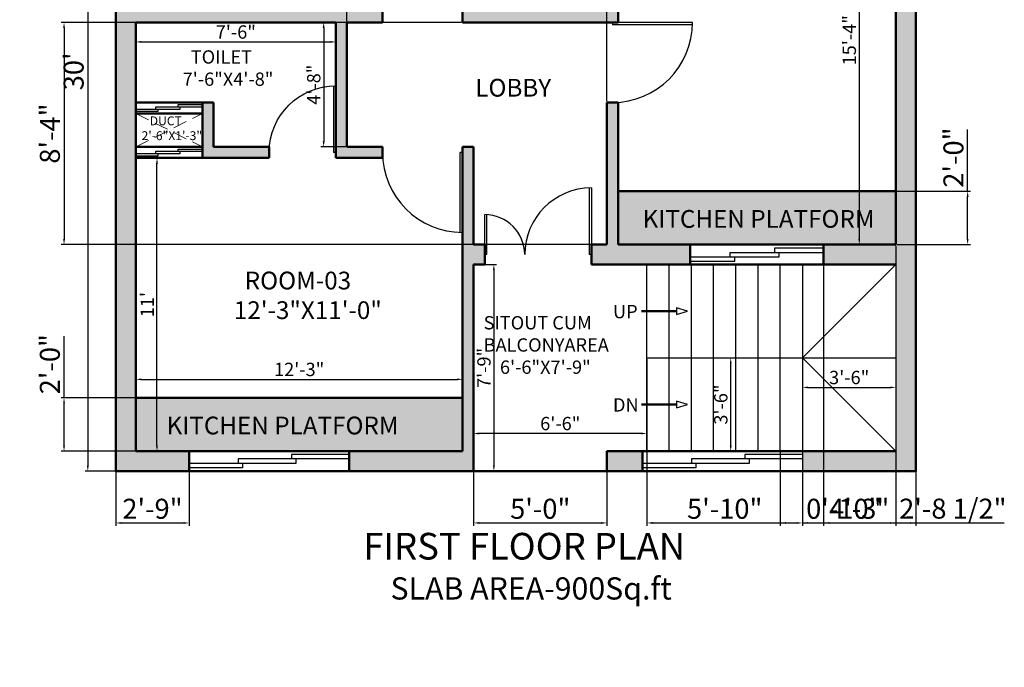
# Model space of a CAD drawing. Units: inches. Extents: x 3274 to 5176, y 1085 to 2172.
# Tile 15 of 16: x 4733 to 5176, y 1085 to 1377. Entities that reach past the tile are written whole.
import ezdxf

# ---------------------------------------------------------------- set-up
doc = ezdxf.new("R2010")
doc.units = ezdxf.units.IN
doc.linetypes.add('DASHED', pattern=[19.05, 12.7, -6.35])
for name, color, linetype, lineweight in [('A-ANNO-DIMS', 2, 'Continuous', 18), ('A-ANNO-TEXT', 7, 'Continuous', 25), ('A-AREA-IDEN', 3, 'Continuous', 25), ('A-DOOR', 4, 'Continuous', 25), ('A-FLOR-OPEN', 7, 'DASHED', 18), ('A-FLOR-PATT', 252, 'Continuous', 13), ('A-FLOR-STRS', 7, 'Continuous', 25), ('A-GLAZ', 5, 'Continuous', 25), ('A-WALL', 7, 'Continuous', 50), ('A-WALL-PATT', 8, 'Continuous', 13)]:
    doc.layers.add(name, color=color, linetype=linetype, lineweight=lineweight)
doc.styles.get("Standard").update_dxf_attribs({"font": 'arial.ttf'})
doc.dimstyles.new('ISO-25', dxfattribs={"dimtxt": 9, "dimasz": 2.5, "dimexe": 1.25, "dimexo": 0.625, "dimtad": 1, "dimdec": 1, "dimlunit": 3, "dimtxsty": 'Standard', "dimcen": 2.5, "dimclrd": 4, "dimclre": 4, "dimclrt": 1, "dimadec": 0, "dimazin": 0, "dimtfac": 1, "dimtdec": 1, "dimtmove": 0, "dimatfit": 3, "dimfxl": 1, "dimarcsym": 0})

# ---------------------------------------------------------------- blocks, each defined once
blk = doc.blocks.new('*D5')
at = {"layer": 'A-ANNO-DIMS', "color": 0, "lineweight": -2, "transparency": 16777216}
for p, q in [((4775.16, 1533.35), (4761.93, 1533.35)), ((4763.18, 1530.85), (4763.18, 1175.85)), ((4775.16, 1173.35), (4761.93, 1173.35))]:
    blk.add_line(p, q, dxfattribs=at)
at = {"layer": 'A-ANNO-DIMS', "color": 0, "transparency": 16777216}
for points in [[(4762.76, 1530.85), (4763.6, 1530.85), (4763.18, 1533.35)], [(4762.76, 1175.85), (4763.6, 1175.85), (4763.18, 1173.35)]]:
    blk.add_solid(points, dxfattribs=at)
at = {"layer": 'Defpoints', "color": 0, "transparency": 16777216}
for p in [(4775.78, 1533.35), (4763.18, 1173.35), (4775.78, 1173.35)]:
    blk.add_point(p, dxfattribs=at)
at = {"layer": 'A-ANNO-DIMS', "color": 0, "transparency": 16777216, "insert": (4757.96, 1353.35), "char_height": 9, "attachment_point": 5, "rotation": 90}
blk.add_mtext("30'", dxfattribs=at)
blk = doc.blocks.new('3')
for p, q in [((47, 30), (47, 0)), ((48, 30), (48, 0)), ((0, 0), (0, 18)), ((1, 0), (1, 18)), ((1, 0), (0, 0)), ((48, 0), (47, 0))]:
    blk.add_line(p, q)
for centre, radius, start, end in [((48, 0), 30, 90, 180), ((0, 0), 18, 0, 90)]:
    blk.add_arc(centre, radius, start, end)
blk = doc.blocks.new('1')
for p, q in [((0, 36), (0, 0)), ((1, 36), (1, 0)), ((0, 0), (1, 0))]:
    blk.add_line(p, q)
blk.add_arc((0, 0), 36, 0, 90)
blk = doc.blocks.new('2')
for p, q in [((0, 30), (0, 0)), ((1, 30), (1, 0)), ((0, 0), (1, 0))]:
    blk.add_line(p, q)
blk.add_arc((0, 0), 30, 0, 90)
blk = doc.blocks.new('*D89')
at = {"layer": 'A-ANNO-DIMS', "color": 0, "lineweight": -2, "transparency": 16777216}
for p, q in [((4784.78, 1206.98), (4784.78, 1215.95)), ((4787.28, 1214.7), (4929.28, 1214.7)), ((4931.78, 1206.98), (4931.78, 1215.95))]:
    blk.add_line(p, q, dxfattribs=at)
at = {"layer": 'A-ANNO-DIMS', "color": 0, "transparency": 16777216}
for points in [[(4787.28, 1215.11), (4787.28, 1214.28), (4784.78, 1214.7)], [(4929.28, 1215.11), (4929.28, 1214.28), (4931.78, 1214.7)]]:
    blk.add_solid(points, dxfattribs=at)
at = {"layer": 'Defpoints', "color": 0, "transparency": 16777216}
for p in [(4931.78, 1214.7), (4784.78, 1206.35), (4931.78, 1206.35)]:
    blk.add_point(p, dxfattribs=at)
at = {"layer": 'A-ANNO-DIMS', "color": 0, "transparency": 16777216, "insert": (4858.28, 1218.39), "char_height": 6, "attachment_point": 5}
blk.add_mtext('12\'-3"', dxfattribs=at)
blk = doc.blocks.new('*D90')
at = {"layer": 'A-ANNO-DIMS', "color": 0, "lineweight": -2, "transparency": 16777216}
for p, q in [((4785.41, 1314.35), (4795.56, 1314.35)), ((4794.31, 1184.85), (4794.31, 1311.85)), ((4785.41, 1182.35), (4795.56, 1182.35))]:
    blk.add_line(p, q, dxfattribs=at)
at = {"layer": 'A-ANNO-DIMS', "color": 0, "transparency": 16777216}
for points in [[(4793.89, 1311.85), (4794.72, 1311.85), (4794.31, 1314.35)], [(4793.89, 1184.85), (4794.72, 1184.85), (4794.31, 1182.35)]]:
    blk.add_solid(points, dxfattribs=at)
at = {"layer": 'Defpoints', "color": 0, "transparency": 16777216}
for p in [(4784.78, 1314.35), (4794.31, 1314.35), (4784.78, 1182.35)]:
    blk.add_point(p, dxfattribs=at)
at = {"layer": 'A-ANNO-DIMS', "color": 0, "transparency": 16777216, "insert": (4790.67, 1248.35), "char_height": 6, "attachment_point": 5, "rotation": 90}
blk.add_mtext("11'", dxfattribs=at)
blk = doc.blocks.new('*D91')
at = {"layer": 'A-ANNO-DIMS', "color": 0, "lineweight": -2, "transparency": 16777216}
for p, q in [((4784.78, 1374.73), (4784.78, 1365.34)), ((4874.78, 1374.73), (4874.78, 1365.34)), ((4787.28, 1366.59), (4872.28, 1366.59))]:
    blk.add_line(p, q, dxfattribs=at)
at = {"layer": 'A-ANNO-DIMS', "color": 0, "transparency": 16777216}
for points in [[(4787.28, 1367.01), (4787.28, 1366.18), (4784.78, 1366.59)], [(4872.28, 1367.01), (4872.28, 1366.18), (4874.78, 1366.59)]]:
    blk.add_solid(points, dxfattribs=at)
at = {"layer": 'Defpoints', "color": 0, "transparency": 16777216}
for p in [(4784.78, 1375.35), (4874.78, 1375.35), (4874.78, 1366.59)]:
    blk.add_point(p, dxfattribs=at)
at = {"layer": 'A-ANNO-DIMS', "color": 0, "transparency": 16777216, "insert": (4829.78, 1370.28), "char_height": 6, "attachment_point": 5}
blk.add_mtext('7\'-6"', dxfattribs=at)
blk = doc.blocks.new('*D92')
at = {"layer": 'A-ANNO-DIMS', "color": 0, "lineweight": -2, "transparency": 16777216}
for p, q in [((4874.16, 1375.35), (4868.06, 1375.35)), ((4869.31, 1372.85), (4869.31, 1321.85)), ((4879.16, 1319.35), (4868.06, 1319.35))]:
    blk.add_line(p, q, dxfattribs=at)
at = {"layer": 'A-ANNO-DIMS', "color": 0, "transparency": 16777216}
for points in [[(4868.89, 1372.85), (4869.73, 1372.85), (4869.31, 1375.35)], [(4868.89, 1321.85), (4869.73, 1321.85), (4869.31, 1319.35)]]:
    blk.add_solid(points, dxfattribs=at)
at = {"layer": 'Defpoints', "color": 0, "transparency": 16777216}
for p in [(4874.78, 1375.35), (4869.31, 1319.35), (4879.78, 1319.35)]:
    blk.add_point(p, dxfattribs=at)
at = {"layer": 'A-ANNO-DIMS', "color": 0, "transparency": 16777216, "insert": (4865.62, 1347.35), "char_height": 6, "attachment_point": 5, "rotation": 90}
blk.add_mtext('4\'-8"', dxfattribs=at)
blk = doc.blocks.new('*D98')
at = {"layer": 'A-ANNO-DIMS', "color": 0, "lineweight": -2, "transparency": 16777216}
for p, q in [((5091.41, 1459.35), (5111.56, 1459.35)), ((5110.31, 1456.85), (5110.31, 1277.85)), ((5091.41, 1275.35), (5111.56, 1275.35))]:
    blk.add_line(p, q, dxfattribs=at)
at = {"layer": 'A-ANNO-DIMS', "color": 0, "transparency": 16777216}
for points in [[(5109.9, 1456.85), (5110.73, 1456.85), (5110.31, 1459.35)], [(5109.9, 1277.85), (5110.73, 1277.85), (5110.31, 1275.35)]]:
    blk.add_solid(points, dxfattribs=at)
at = {"layer": 'Defpoints', "color": 0, "transparency": 16777216}
for p in [(5090.78, 1459.35), (5090.78, 1275.35), (5110.31, 1275.35)]:
    blk.add_point(p, dxfattribs=at)
at = {"layer": 'A-ANNO-DIMS', "color": 0, "transparency": 16777216, "insert": (5106.62, 1367.35), "char_height": 6, "attachment_point": 5, "rotation": 90}
blk.add_mtext('15\'-4"', dxfattribs=at)
blk = doc.blocks.new('*D104')
at = {"layer": 'A-ANNO-DIMS', "color": 0, "lineweight": -2, "transparency": 16777216}
for p, q in [((4937.41, 1266.35), (4947.14, 1266.35)), ((4945.89, 1263.85), (4945.89, 1175.85)), ((4937.41, 1173.35), (4947.14, 1173.35))]:
    blk.add_line(p, q, dxfattribs=at)
at = {"layer": 'A-ANNO-DIMS', "color": 0, "transparency": 16777216}
for points in [[(4945.48, 1263.85), (4946.31, 1263.85), (4945.89, 1266.35)], [(4945.48, 1175.85), (4946.31, 1175.85), (4945.89, 1173.35)]]:
    blk.add_solid(points, dxfattribs=at)
at = {"layer": 'Defpoints', "color": 0, "transparency": 16777216}
for p in [(4936.78, 1266.35), (4936.78, 1173.35), (4945.89, 1173.35)]:
    blk.add_point(p, dxfattribs=at)
at = {"layer": 'A-ANNO-DIMS', "color": 0, "transparency": 16777216, "insert": (4942.21, 1219.85), "char_height": 6, "attachment_point": 5, "rotation": 90}
blk.add_mtext('7\'-9"', dxfattribs=at)
blk = doc.blocks.new('*D105')
at = {"layer": 'A-ANNO-DIMS', "color": 0, "lineweight": -2, "transparency": 16777216}
for p, q in [((4936.78, 1190.96), (4936.78, 1191.58)), ((5012.28, 1190.33), (4939.28, 1190.33)), ((5014.78, 1190.96), (5014.78, 1191.58))]:
    blk.add_line(p, q, dxfattribs=at)
at = {"layer": 'A-ANNO-DIMS', "color": 0, "transparency": 16777216}
for points in [[(4939.28, 1190.75), (4939.28, 1189.92), (4936.78, 1190.33)], [(5012.28, 1190.75), (5012.28, 1189.92), (5014.78, 1190.33)]]:
    blk.add_solid(points, dxfattribs=at)
at = {"layer": 'Defpoints', "color": 0, "transparency": 16777216}
for p in [(4936.78, 1190.33), (4936.78, 1190.33), (5014.78, 1190.33)]:
    blk.add_point(p, dxfattribs=at)
at = {"layer": 'A-ANNO-DIMS', "color": 0, "transparency": 16777216, "insert": (4975.78, 1194.02), "char_height": 6, "attachment_point": 5}
blk.add_mtext('6\'-6"', dxfattribs=at)
blk = doc.blocks.new('*D106')
at = {"layer": 'A-ANNO-DIMS', "color": 0, "lineweight": -2, "transparency": 16777216}
for p, q in [((5050.97, 1224.35), (5053.72, 1224.35)), ((5052.47, 1184.85), (5052.47, 1221.85)), ((5050.97, 1182.35), (5053.72, 1182.35))]:
    blk.add_line(p, q, dxfattribs=at)
at = {"layer": 'A-ANNO-DIMS', "color": 0, "transparency": 16777216}
for points in [[(5052.06, 1221.85), (5052.89, 1221.85), (5052.47, 1224.35)], [(5052.06, 1184.85), (5052.89, 1184.85), (5052.47, 1182.35)]]:
    blk.add_solid(points, dxfattribs=at)
at = {"layer": 'Defpoints', "color": 0, "transparency": 16777216}
for p in [(5050.35, 1224.35), (5052.47, 1224.35), (5050.35, 1182.35)]:
    blk.add_point(p, dxfattribs=at)
at = {"layer": 'A-ANNO-DIMS', "color": 0, "transparency": 16777216, "insert": (5048.78, 1203.35), "char_height": 6, "attachment_point": 5, "rotation": 90}
blk.add_mtext('3\'-6"', dxfattribs=at)
blk = doc.blocks.new('*D107')
at = {"layer": 'A-ANNO-DIMS', "color": 0, "lineweight": -2, "transparency": 16777216}
for p, q in [((5084.78, 1213.78), (5084.78, 1209.81)), ((5087.28, 1211.06), (5124.28, 1211.06)), ((5126.78, 1213.78), (5126.78, 1209.81))]:
    blk.add_line(p, q, dxfattribs=at)
at = {"layer": 'A-ANNO-DIMS', "color": 0, "transparency": 16777216}
for points in [[(5087.28, 1211.47), (5087.28, 1210.64), (5084.78, 1211.06)], [(5124.28, 1211.47), (5124.28, 1210.64), (5126.78, 1211.06)]]:
    blk.add_solid(points, dxfattribs=at)
at = {"layer": 'Defpoints', "color": 0, "transparency": 16777216}
for p in [(5084.78, 1214.41), (5126.78, 1214.41), (5126.78, 1211.06)]:
    blk.add_point(p, dxfattribs=at)
at = {"layer": 'A-ANNO-DIMS', "color": 0, "transparency": 16777216, "insert": (5105.78, 1214.75), "char_height": 6, "attachment_point": 5}
blk.add_mtext('3\'-6"', dxfattribs=at)
blk = doc.blocks.new('WIN-30')
for p, q in [((4366.19, 1316.35), (4386.19, 1316.35)), ((4375.19, 1317.35), (4396.19, 1317.35)), ((4375.19, 1316.35), (4375.19, 1317.35)), ((4376.19, 1315.35), (4376.19, 1316.35)), ((4385.19, 1318.35), (4396.19, 1318.35)), ((4385.19, 1317.35), (4385.19, 1318.35)), ((4386.19, 1316.35), (4386.19, 1317.35)), ((4366.19, 1315.35), (4376.19, 1315.35))]:
    blk.add_line(p, q)
blk = doc.blocks.new('WIN-60')
for p, q in [((4598.19, 1271.85), (4640.19, 1271.85)), ((4598.19, 1269.85), (4598.19, 1271.85)), ((4618.19, 1273.85), (4640.19, 1273.85)), ((4618.19, 1271.85), (4618.19, 1273.85)), ((4620.19, 1269.85), (4620.19, 1271.85)), ((4580.19, 1269.85), (4620.19, 1269.85)), ((4580.19, 1267.85), (4600.19, 1267.85)), ((4600.19, 1267.85), (4600.19, 1269.85))]:
    blk.add_line(p, q)
blk = doc.blocks.new('WIN-72')
for p, q in [((4462.19, 1178.85), (4412.19, 1178.85)), ((4412.19, 1178.85), (4412.19, 1176.85)), ((4462.19, 1180.85), (4436.19, 1180.85)), ((4436.19, 1180.85), (4436.19, 1178.85)), ((4438.19, 1178.85), (4438.19, 1176.85)), ((4438.19, 1176.85), (4390.19, 1176.85)), ((4414.19, 1174.85), (4390.19, 1174.85)), ((4414.19, 1176.85), (4414.19, 1174.85))]:
    blk.add_line(p, q)
blk = doc.blocks.new('*D136')
at = {"layer": 'A-ANNO-DIMS', "color": 4, "lineweight": -2, "transparency": 16777216}
for p, q in [((4708.83, 1369.73), (4723.61, 1369.73)), ((4722.36, 1367.23), (4722.36, 1277.84)), ((4708.83, 1275.34), (4723.61, 1275.34)), ((4722.36, 1275.34), (4722.36, 1085.06))]:
    blk.add_line(p, q, dxfattribs=at)
at = {"layer": 'A-ANNO-DIMS', "color": 4, "transparency": 16777216}
for points in [[(4721.94, 1367.23), (4722.78, 1367.23), (4722.36, 1369.73)], [(4721.94, 1277.84), (4722.78, 1277.84), (4722.36, 1275.34)]]:
    blk.add_solid(points, dxfattribs=at)
at = {"layer": 'Defpoints', "color": 0, "transparency": 16777216}
for p in [(4708.2, 1369.73), (4708.2, 1275.34), (4722.36, 1275.34)]:
    blk.add_point(p, dxfattribs=at)
at = {"layer": 'A-ANNO-DIMS', "color": 1, "transparency": 16777216, "insert": (4717.08, 1178.95), "char_height": 9, "attachment_point": 5, "rotation": 90}
blk.add_mtext('L-SHAPED SOFA 7\'-10 1/2" TYP.', dxfattribs=at)
blk = doc.blocks.new('*D137')
at = {"layer": 'A-ANNO-DIMS', "color": 4, "lineweight": -2, "transparency": 16777216}
for p, q in [((4654.05, 1370.36), (4654.05, 1385.14)), ((4656.55, 1383.89), (4705.7, 1383.89)), ((4708.2, 1370.36), (4708.2, 1385.14)), ((4708.2, 1383.89), (4767.17, 1383.89))]:
    blk.add_line(p, q, dxfattribs=at)
at = {"layer": 'A-ANNO-DIMS', "color": 4, "transparency": 16777216}
for points in [[(4656.55, 1384.31), (4656.55, 1383.47), (4654.05, 1383.89)], [(4705.7, 1384.31), (4705.7, 1383.47), (4708.2, 1383.89)]]:
    blk.add_solid(points, dxfattribs=at)
at = {"layer": 'Defpoints', "color": 0, "transparency": 16777216}
for p in [(4708.2, 1383.89), (4654.05, 1369.73), (4708.2, 1369.73)]:
    blk.add_point(p, dxfattribs=at)
at = {"layer": 'A-ANNO-DIMS', "color": 1, "transparency": 16777216, "insert": (4738.94, 1389.11), "char_height": 9, "attachment_point": 5}
blk.add_mtext('4\'-6" TYP.', dxfattribs=at)
blk = doc.blocks.new('*D180')
at = {"layer": 'A-ANNO-DIMS', "color": 4, "lineweight": -2, "transparency": 16777216}
for p, q in [((4775.78, 1172.73), (4775.78, 1148.8)), ((4808.78, 1172.73), (4808.78, 1148.8)), ((4778.28, 1150.05), (4806.28, 1150.05))]:
    blk.add_line(p, q, dxfattribs=at)
at = {"layer": 'A-ANNO-DIMS', "color": 4, "transparency": 16777216}
for points in [[(4778.28, 1150.47), (4778.28, 1149.64), (4775.78, 1150.05)], [(4806.28, 1150.47), (4806.28, 1149.64), (4808.78, 1150.05)]]:
    blk.add_solid(points, dxfattribs=at)
at = {"layer": 'Defpoints', "color": 0, "transparency": 16777216}
for p in [(4775.78, 1173.35), (4808.78, 1173.35), (4808.78, 1150.05)]:
    blk.add_point(p, dxfattribs=at)
at = {"layer": 'A-ANNO-DIMS', "color": 1, "transparency": 16777216, "insert": (4792.28, 1155.27), "char_height": 9, "attachment_point": 5}
blk.add_mtext('2\'-9"', dxfattribs=at)
blk = doc.blocks.new('*D181')
at = {"layer": 'A-ANNO-DIMS', "color": 4, "lineweight": -2, "transparency": 16777216}
for p, q in [((5084.78, 1172.73), (5084.78, 1148.8)), ((5135.78, 1172.73), (5135.78, 1148.8)), ((5087.28, 1150.05), (5133.28, 1150.05))]:
    blk.add_line(p, q, dxfattribs=at)
at = {"layer": 'A-ANNO-DIMS', "color": 4, "transparency": 16777216}
for points in [[(5087.28, 1150.47), (5087.28, 1149.64), (5084.78, 1150.05)], [(5133.28, 1150.47), (5133.28, 1149.64), (5135.78, 1150.05)]]:
    blk.add_solid(points, dxfattribs=at)
at = {"layer": 'Defpoints', "color": 0, "transparency": 16777216}
for p in [(5084.78, 1173.35), (5135.78, 1173.35), (5135.78, 1150.05)]:
    blk.add_point(p, dxfattribs=at)
at = {"layer": 'A-ANNO-DIMS', "color": 1, "transparency": 16777216, "insert": (5110.28, 1155.28), "char_height": 9, "attachment_point": 5}
blk.add_mtext('4\'-3"', dxfattribs=at)
blk = doc.blocks.new('*D182')
at = {"layer": 'A-ANNO-DIMS', "color": 4, "lineweight": -2, "transparency": 16777216}
for p, q in [((4936.78, 1172.73), (4936.78, 1148.8)), ((4996.78, 1172.73), (4996.78, 1148.8)), ((4939.28, 1150.05), (4994.28, 1150.05))]:
    blk.add_line(p, q, dxfattribs=at)
at = {"layer": 'A-ANNO-DIMS', "color": 4, "transparency": 16777216}
for points in [[(4939.28, 1150.47), (4939.28, 1149.64), (4936.78, 1150.05)], [(4994.28, 1150.47), (4994.28, 1149.64), (4996.78, 1150.05)]]:
    blk.add_solid(points, dxfattribs=at)
at = {"layer": 'Defpoints', "color": 0, "transparency": 16777216}
for p in [(4936.78, 1173.35), (4996.78, 1173.35), (4996.78, 1150.05)]:
    blk.add_point(p, dxfattribs=at)
at = {"layer": 'A-ANNO-DIMS', "color": 1, "transparency": 16777216, "insert": (4966.78, 1155.27), "char_height": 9, "attachment_point": 5}
blk.add_mtext('5\'-0"', dxfattribs=at)
blk = doc.blocks.new('*D183')
at = {"layer": 'A-ANNO-DIMS', "color": 4, "lineweight": -2, "transparency": 16777216}
for p, q in [((4752.48, 1206.35), (4752.48, 1234.18)), ((4931.16, 1206.35), (4751.23, 1206.35)), ((4752.48, 1184.85), (4752.48, 1203.85)), ((4931.16, 1182.35), (4751.23, 1182.35))]:
    blk.add_line(p, q, dxfattribs=at)
at = {"layer": 'A-ANNO-DIMS', "color": 4, "transparency": 16777216}
for points in [[(4752.07, 1203.85), (4752.9, 1203.85), (4752.48, 1206.35)], [(4752.07, 1184.85), (4752.9, 1184.85), (4752.48, 1182.35)]]:
    blk.add_solid(points, dxfattribs=at)
at = {"layer": 'Defpoints', "color": 0, "transparency": 16777216}
for p in [(4752.48, 1206.35), (4931.78, 1206.35), (4931.78, 1182.35)]:
    blk.add_point(p, dxfattribs=at)
at = {"layer": 'A-ANNO-DIMS', "color": 1, "transparency": 16777216, "insert": (4747.26, 1221.52), "char_height": 9, "attachment_point": 5, "rotation": 90}
blk.add_mtext('2\'-0"', dxfattribs=at)
blk = doc.blocks.new('*D185')
at = {"layer": 'A-ANNO-DIMS', "color": 4, "lineweight": -2, "transparency": 16777216}
for p, q in [((5159.08, 1299.35), (5159.08, 1327.18)), ((5127.41, 1299.35), (5160.33, 1299.35)), ((5159.08, 1277.85), (5159.08, 1296.85)), ((5127.41, 1275.35), (5160.33, 1275.35))]:
    blk.add_line(p, q, dxfattribs=at)
at = {"layer": 'A-ANNO-DIMS', "color": 4, "transparency": 16777216}
for points in [[(5158.67, 1296.85), (5159.5, 1296.85), (5159.08, 1299.35)], [(5158.67, 1277.85), (5159.5, 1277.85), (5159.08, 1275.35)]]:
    blk.add_solid(points, dxfattribs=at)
at = {"layer": 'Defpoints', "color": 0, "transparency": 16777216}
for p in [(5126.78, 1299.35), (5159.08, 1299.35), (5126.78, 1275.35)]:
    blk.add_point(p, dxfattribs=at)
at = {"layer": 'A-ANNO-DIMS', "color": 1, "transparency": 16777216, "insert": (5153.86, 1314.52), "char_height": 9, "attachment_point": 5, "rotation": 90}
blk.add_mtext('2\'-0"', dxfattribs=at)
blk = doc.blocks.new('*D186')
at = {"layer": 'A-ANNO-DIMS', "color": 4, "lineweight": -2, "transparency": 16777216}
for p, q in [((5014.78, 1223.73), (5014.78, 1148.8)), ((5084.78, 1223.73), (5084.78, 1148.8)), ((5017.28, 1150.05), (5082.28, 1150.05))]:
    blk.add_line(p, q, dxfattribs=at)
at = {"layer": 'A-ANNO-DIMS', "color": 4, "transparency": 16777216}
for points in [[(5017.28, 1150.47), (5017.28, 1149.64), (5014.78, 1150.05)], [(5082.28, 1150.47), (5082.28, 1149.64), (5084.78, 1150.05)]]:
    blk.add_solid(points, dxfattribs=at)
at = {"layer": 'Defpoints', "color": 0, "transparency": 16777216}
for p in [(5014.78, 1224.35), (5084.78, 1224.35), (5084.78, 1150.05)]:
    blk.add_point(p, dxfattribs=at)
at = {"layer": 'A-ANNO-DIMS', "color": 1, "transparency": 16777216, "insert": (5049.78, 1155.27), "char_height": 9, "attachment_point": 5}
blk.add_mtext('5\'-10"', dxfattribs=at)
blk = doc.blocks.new('*D187')
at = {"layer": 'A-ANNO-DIMS', "color": 4, "lineweight": -2, "transparency": 16777216}
for p, q in [((5074.78, 1181.73), (5074.78, 1148.8)), ((5084.78, 1181.73), (5084.78, 1148.8)), ((5077.28, 1150.05), (5082.28, 1150.05)), ((5084.78, 1150.05), (5119.45, 1150.05))]:
    blk.add_line(p, q, dxfattribs=at)
at = {"layer": 'A-ANNO-DIMS', "color": 4, "transparency": 16777216}
for points in [[(5077.28, 1150.47), (5077.28, 1149.64), (5074.78, 1150.05)], [(5082.28, 1150.47), (5082.28, 1149.64), (5084.78, 1150.05)]]:
    blk.add_solid(points, dxfattribs=at)
at = {"layer": 'Defpoints', "color": 0, "transparency": 16777216}
for p in [(5074.78, 1182.35), (5084.78, 1182.35), (5084.78, 1150.05)]:
    blk.add_point(p, dxfattribs=at)
at = {"layer": 'A-ANNO-DIMS', "color": 1, "transparency": 16777216, "insert": (5103.37, 1155.27), "char_height": 9, "attachment_point": 5}
blk.add_mtext('0\'-10"', dxfattribs=at)
blk = doc.blocks.new('*D188')
at = {"layer": 'A-ANNO-DIMS', "color": 4, "lineweight": -2, "transparency": 16777216}
for p, q in [((4879.78, 1375.98), (4879.78, 1557.9)), ((4882.28, 1556.65), (4994.28, 1556.65)), ((4996.78, 1339.98), (4996.78, 1557.9))]:
    blk.add_line(p, q, dxfattribs=at)
at = {"layer": 'A-ANNO-DIMS', "color": 4, "transparency": 16777216}
for points in [[(4882.28, 1557.07), (4882.28, 1556.24), (4879.78, 1556.65)], [(4994.28, 1557.07), (4994.28, 1556.24), (4996.78, 1556.65)]]:
    blk.add_solid(points, dxfattribs=at)
at = {"layer": 'Defpoints', "color": 0, "transparency": 16777216}
for p in [(4996.78, 1556.65), (4879.78, 1375.35), (4996.78, 1339.35)]:
    blk.add_point(p, dxfattribs=at)
at = {"layer": 'A-ANNO-DIMS', "color": 1, "transparency": 16777216, "insert": (4938.28, 1561.87), "char_height": 9, "attachment_point": 5}
blk.add_mtext('9\'-9"', dxfattribs=at)
blk = doc.blocks.new('*D189')
at = {"layer": 'A-ANNO-DIMS', "color": 4, "lineweight": -2, "transparency": 16777216}
for p, q in [((4931.16, 1375.35), (4751.23, 1375.35)), ((4752.48, 1372.85), (4752.48, 1277.85)), ((4996.16, 1275.35), (4751.23, 1275.35))]:
    blk.add_line(p, q, dxfattribs=at)
at = {"layer": 'A-ANNO-DIMS', "color": 4, "transparency": 16777216}
for points in [[(4752.07, 1372.85), (4752.9, 1372.85), (4752.48, 1375.35)], [(4752.07, 1277.85), (4752.9, 1277.85), (4752.48, 1275.35)]]:
    blk.add_solid(points, dxfattribs=at)
at = {"layer": 'Defpoints', "color": 0, "transparency": 16777216}
for p in [(4931.78, 1375.35), (4752.48, 1275.35), (4996.78, 1275.35)]:
    blk.add_point(p, dxfattribs=at)
at = {"layer": 'A-ANNO-DIMS', "color": 1, "transparency": 16777216, "insert": (4747.26, 1325.35), "char_height": 9, "attachment_point": 5, "rotation": 90}
blk.add_mtext('8\'-4"', dxfattribs=at)
blk = doc.blocks.new('*D190')
at = {"layer": 'A-ANNO-DIMS', "color": 4, "lineweight": -2, "transparency": 16777216}
for p, q in [((5094.28, 1274.73), (5094.28, 1148.8)), ((5126.78, 1274.73), (5126.78, 1148.8)), ((5096.78, 1150.05), (5124.28, 1150.05)), ((5126.78, 1150.05), (5175.58, 1150.05))]:
    blk.add_line(p, q, dxfattribs=at)
at = {"layer": 'A-ANNO-DIMS', "color": 4, "transparency": 16777216}
for points in [[(5096.78, 1150.47), (5096.78, 1149.64), (5094.28, 1150.05)], [(5124.28, 1150.47), (5124.28, 1149.64), (5126.78, 1150.05)]]:
    blk.add_solid(points, dxfattribs=at)
at = {"layer": 'Defpoints', "color": 0, "transparency": 16777216}
for p in [(5094.28, 1275.35), (5126.78, 1275.35), (5126.78, 1150.05)]:
    blk.add_point(p, dxfattribs=at)
at = {"layer": 'A-ANNO-DIMS', "color": 1, "transparency": 16777216, "insert": (5152.43, 1155.33), "char_height": 9, "attachment_point": 5}
blk.add_mtext('2\'-8 1/2"', dxfattribs=at)

msp = doc.modelspace()

# ---------------------------------------------------------------- hatches: boundary and pattern name
at = {"layer": 'A-FLOR-PATT'}
h = msp.add_hatch(color=256, dxfattribs=at)
h.dxf.hatch_style = 1
h.paths.add_polyline_path([(5001.78, 1275.35), (5126.78, 1275.35), (5126.78, 1299.35), (5001.78, 1299.35)])
h.paths.add_polyline_path([(5010.01, 1278.41), (5127.02, 1278.41), (5127.02, 1294.9), (5010.01, 1294.9)], flags=9)
h = msp.add_hatch(color=256, dxfattribs=at)
h.dxf.hatch_style = 1
h.paths.add_polyline_path([(4784.78, 1206.35), (4784.78, 1182.35), (4931.78, 1182.35), (4931.78, 1206.35)])
h.paths.add_polyline_path([(4795.81, 1185.41), (4912.82, 1185.41), (4912.82, 1201.9), (4795.81, 1201.9)], flags=24)
at = {"layer": 'A-WALL-PATT'}
h = msp.add_hatch(color=256, dxfattribs=at)
h.dxf.hatch_style = 1
h.paths.add_polyline_path([(4819.78, 1319.35), (4819.78, 1339.35), (4814.78, 1339.35), (4814.78, 1314.35), (4844.78, 1314.35), (4844.78, 1319.35)], flags=17)
h.paths.add_polyline_path([(4775.78, 1173.35), (4808.78, 1173.35), (4808.78, 1182.35), (4784.78, 1182.35), (4784.78, 1375.35), (4874.78, 1375.35), (4874.78, 1314.35), (4895.78, 1314.35), (4895.78, 1319.35), (4879.78, 1319.35), (4879.78, 1375.35), (4895.78, 1375.35), (4895.78, 1380.35), (4784.78, 1380.35), (4784.78, 1524.35), (5085.78, 1524.35), (5085.78, 1494.35), (5090.78, 1494.35), (5090.78, 1524.35), (5126.78, 1524.35), (5126.78, 1275.35), (5094.28, 1275.35), (5094.28, 1266.35), (5126.78, 1266.35), (5126.78, 1182.35), (5084.78, 1182.35), (5084.78, 1173.35), (5135.78, 1173.35), (5135.78, 1533.35), (4775.78, 1533.35)])
h.paths.add_polyline_path([(4996.78, 1380.35), (4936.78, 1380.35), (4936.78, 1418.35), (4934.28, 1418.35), (4931.78, 1418.35), (4931.78, 1375.35), (5001.78, 1375.35), (5001.78, 1459.35), (5090.78, 1459.35), (5090.78, 1464.35), (5001.78, 1464.35), (5001.78, 1488.35), (4978.78, 1488.35), (4978.78, 1483.35), (4996.78, 1483.35)], flags=17)
h.paths.add_polyline_path([(4931.78, 1488.35), (4931.78, 1448.35), (4936.78, 1448.35), (4936.78, 1483.35), (4954.78, 1483.35), (4954.78, 1488.35)], flags=17)
h.paths.add_polyline_path([(5034.28, 1266.35), (5034.28, 1275.35), (5001.78, 1275.35), (5001.78, 1339.35), (4996.78, 1339.35), (4996.78, 1275.35), (4989.78, 1275.35), (4989.78, 1270.85), (4989.78, 1266.35)], flags=17)
h.paths.add_polyline_path([(4936.78, 1266.35), (4941.78, 1266.35), (4941.78, 1275.35), (4936.78, 1275.35), (4936.78, 1319.35), (4931.78, 1319.35), (4931.78, 1182.35), (4880.78, 1182.35), (4880.78, 1173.35), (4936.78, 1173.35)], flags=17)
h.paths.add_polyline_path([(4996.78, 1182.35), (4996.78, 1173.35), (5012.78, 1173.35), (5012.78, 1182.35)], flags=17)

# ---------------------------------------------------------------- linework, layer by layer
at = {"layer": 'A-FLOR-OPEN', "ltscale": 0.5}
for p, q in [((4784.78, 1334.35), (4814.78, 1319.35)), ((4784.78, 1319.35), (4814.78, 1334.35))]:
    msp.add_line(p, q, dxfattribs=at)
at = {"layer": 'A-FLOR-STRS'}
for p, q in [((5014.78, 1224.35), (5014.78, 1266.35)), ((5024.78, 1224.35), (5024.78, 1266.35)), ((5034.78, 1224.35), (5034.78, 1266.35)), ((5044.78, 1224.35), (5044.78, 1266.35)), ((5054.78, 1224.35), (5054.78, 1266.35)), ((5064.78, 1224.35), (5064.78, 1266.35)), ((5074.78, 1224.35), (5074.78, 1266.35)), ((5084.78, 1266.35), (5084.78, 1182.35)), ((5084.78, 1224.35), (5126.78, 1266.35)), ((5126.78, 1266.35), (5126.78, 1182.35)), ((5014.78, 1224.35), (5126.78, 1224.35)), ((5014.78, 1182.35), (5014.78, 1224.35)), ((5024.78, 1182.35), (5024.78, 1224.35)), ((5034.78, 1182.35), (5034.78, 1224.35)), ((5044.78, 1182.35), (5044.78, 1224.35)), ((5054.78, 1182.35), (5054.78, 1224.35)), ((5064.78, 1182.35), (5064.78, 1224.35)), ((5074.78, 1182.35), (5074.78, 1224.35)), ((5084.78, 1224.35), (5126.78, 1182.35)), ((5084.78, 1182.35), (5084.78, 1173.35))]:
    msp.add_line(p, q, dxfattribs=at)
for points in [[(5032.99, 1245.35), (5028.1, 1246.85), (5028.1, 1243.86)], [(5032.99, 1203.35), (5028.1, 1204.85), (5028.1, 1201.86)]]:
    msp.add_lwpolyline(points, close=True, dxfattribs=at)
at = {"layer": 'A-WALL'}
for p, q in [((5126.78, 1524.35), (5126.78, 1275.35)), ((5001.78, 1459.35), (5001.78, 1375.35)), ((4931.78, 1375.35), (4931.78, 1418.35)), ((4895.78, 1375.35), (4895.78, 1380.35)), ((4784.78, 1375.35), (4874.78, 1375.35)), ((4784.78, 1182.35), (4784.78, 1375.35)), ((4874.78, 1314.35), (4874.78, 1375.35)), ((4879.78, 1319.35), (4879.78, 1375.35)), ((4879.78, 1375.35), (4895.78, 1375.35)), ((4931.78, 1375.35), (5001.78, 1375.35)), ((4784.78, 1339.35), (4819.78, 1339.35)), ((4814.78, 1314.35), (4814.78, 1339.35)), ((4819.78, 1319.35), (4819.78, 1339.35)), ((4996.78, 1339.35), (4996.78, 1275.35)), ((4996.78, 1339.35), (5001.78, 1339.35)), ((5001.78, 1339.35), (5001.78, 1275.35)), ((4784.78, 1334.35), (4814.78, 1334.35)), ((4784.78, 1319.35), (4814.78, 1319.35)), ((4819.78, 1319.35), (4844.78, 1319.35)), ((4844.78, 1314.35), (4844.78, 1319.35)), ((4879.78, 1319.35), (4895.78, 1319.35)), ((4895.78, 1314.35), (4895.78, 1319.35)), ((4931.78, 1182.35), (4931.78, 1319.35)), ((4931.78, 1319.35), (4936.78, 1319.35)), ((4936.78, 1275.35), (4936.78, 1319.35)), ((4784.78, 1314.35), (4844.78, 1314.35)), ((4874.78, 1314.35), (4895.78, 1314.35)), ((5001.78, 1299.35), (5126.78, 1299.35)), ((4936.78, 1275.35), (4941.78, 1275.35)), ((4941.78, 1266.35), (4941.78, 1275.35)), ((4989.78, 1275.35), (4996.78, 1275.35)), ((4989.78, 1266.35), (4989.78, 1275.35)), ((5001.78, 1275.35), (5126.78, 1275.35)), ((5034.28, 1266.35), (5034.28, 1275.35)), ((5094.28, 1266.35), (5094.28, 1275.35)), ((4936.78, 1266.35), (4941.78, 1266.35)), ((4936.78, 1173.35), (4936.78, 1266.35)), ((4989.78, 1266.35), (5126.78, 1266.35)), ((5012.34, 1245.35), (5028.1, 1245.35)), ((4931.78, 1206.35), (4784.78, 1206.35)), ((5012.34, 1203.35), (5028.1, 1203.35)), ((4931.78, 1182.35), (4784.78, 1182.35)), ((4808.78, 1182.35), (4808.78, 1173.35)), ((4880.78, 1182.35), (4880.78, 1173.35)), ((5126.78, 1182.35), (4996.78, 1182.35)), ((4996.78, 1173.35), (4996.78, 1182.35)), ((5012.78, 1182.35), (5012.78, 1173.35))]:
    msp.add_line(p, q, dxfattribs=at)
msp.add_lwpolyline([(4936.78, 1173.35), (4775.78, 1173.35), (4775.78, 1533.35), (5135.78, 1533.35), (5135.78, 1173.35), (4936.78, 1173.35)], dxfattribs=at)

# ---------------------------------------------------------------- block references
at = {"layer": 'A-DOOR'}
for p, rotation in [((4999.28, 1375.35), 270), ((4931.78, 1316.85), 180)]:
    msp.add_blockref('1', p, dxfattribs=dict(at, rotation=rotation))
at = {"layer": 'A-DOOR', "xscale": -1}
msp.add_blockref('2', (4874.78, 1316.85), dxfattribs=at)
at = {"layer": 'A-DOOR'}
msp.add_blockref('3', (4941.78, 1270.85), dxfattribs=at)
at = {"layer": 'A-GLAZ'}
for name, p in [('WIN-30', (418.6, 20)), ('WIN-30', (418.6, 0)), ('WIN-60', (454.1, 0)), ('WIN-72', (418.6, 0)), ('WIN-72', (622.6, 0))]:
    msp.add_blockref(name, p, dxfattribs=at)

# ---------------------------------------------------------------- texts
at = {"layer": 'A-ANNO-TEXT'}
for s, p in [('UP', (4999.5, 1242.2)), ('DN', (4999.5, 1200.2))]:
    msp.add_text(s, height=6, dxfattribs=at).set_placement(p)
at = {"layer": 'A-ANNO-TEXT', "insert": (4887.17, 1145.58), "char_height": 12, "attachment_point": 1}
msp.add_mtext_dynamic_manual_height_columns('FIRST FLOOR PLAN\\P{\\H0.83333x;    SLAB AREA-900Sq.ft}', width=202.3193, gutter_width=30, heights=[0], dxfattribs=at)
at = {"layer": 'A-AREA-IDEN', "attachment_point": 1}
for s, width, heights, insert, char_height in [('  TOILET\\P7\'-6"X4\'-8"', 58.0121, [16.24], (4805.85, 1362.83), 6), ('LOBBY', 58.0121, [16.24], (4937.53, 1349.97), 8), ('   DUCT\\P2\'-6"X1\'-3"', 58.0121, [16.24], (4787.38, 1333.06), 4), ('KITCHEN PLATFORM', 147.1149, [0], (5012.83, 1290.92), 8), ('  ROOM-03\\P12\'-3"X11\'-0"', 58.0121, [0], (4828.89, 1263.18), 8), ('SITOUT CUM BALCONYAREA \\P    6\'-6"X7\'-9"', 58.0121, [0], (4941.29, 1243.18), 6), ('KITCHEN PLATFORM', 147.1149, [0], (4798.63, 1197.92), 8)]:
    msp.add_mtext_dynamic_manual_height_columns(s, width=width, gutter_width=30, heights=heights, dxfattribs=dict(at, insert=insert, char_height=char_height))

# ---------------------------------------------------------------- dimensions: what is measured, and where the dimension line sits
at = {"layer": 'A-ANNO-DIMS'}
for base, p1, p2, override, picture, middle in [((4996.78, 1556.65), (4879.78, 1375.35), (4996.78, 1339.35), {"dimdec": 1, "dimlfac": 1, "dimrnd": 0, "dimzin": 1, "dimdsep": 46, "dimlunit": 4, "dimfrac": 2}, '*D188', (4938.28, 1561.87)), ((4874.78, 1366.59), (4784.78, 1375.35), (4874.78, 1375.35), {"dimtxt": 6, "dimclrd": 0, "dimclre": 0, "dimclrt": 0}, '*D91', (4829.78, 1370.28)), ((5126.78, 1150.05), (5094.28, 1275.35), (5126.78, 1275.35), {"dimdec": 1, "dimlfac": 1, "dimrnd": 0, "dimzin": 1, "dimdsep": 46, "dimlunit": 4, "dimfrac": 2}, '*D190', (5152.43, 1155.33)), ((5084.78, 1150.05), (5014.78, 1224.35), (5084.78, 1224.35), {"dimdec": 1, "dimlfac": 1, "dimrnd": 0, "dimzin": 1, "dimdsep": 46, "dimlunit": 4, "dimfrac": 2}, '*D186', (5049.78, 1155.27)), ((4931.78, 1214.7), (4784.78, 1206.35), (4931.78, 1206.35), {"dimtxt": 6, "dimclrd": 0, "dimclre": 0, "dimclrt": 0}, '*D89', (4858.28, 1218.39)), ((5126.78, 1211.06), (5084.78, 1214.41), (5126.78, 1214.41), {"dimtxt": 6, "dimclrd": 0, "dimclre": 0, "dimclrt": 0}, '*D107', (5105.78, 1214.75)), ((4936.78, 1190.33), (5014.78, 1190.33), (4936.78, 1190.33), {"dimtxt": 6, "dimclrd": 0, "dimclre": 0, "dimclrt": 0}, '*D105', (4975.78, 1194.02)), ((5084.78, 1150.05), (5074.78, 1182.35), (5084.78, 1182.35), {"dimdec": 1, "dimlfac": 1, "dimrnd": 0, "dimzin": 1, "dimdsep": 46, "dimlunit": 4, "dimfrac": 2}, '*D187', (5103.37, 1155.27)), ((4808.78, 1150.05), (4775.78, 1173.35), (4808.78, 1173.35), {"dimdec": 1, "dimlfac": 1, "dimrnd": 0, "dimzin": 1, "dimdsep": 46, "dimlunit": 4, "dimfrac": 2}, '*D180', (4792.28, 1155.27)), ((4996.78, 1150.05), (4936.78, 1173.35), (4996.78, 1173.35), {"dimdec": 1, "dimlfac": 1, "dimrnd": 0, "dimzin": 1, "dimdsep": 46, "dimlunit": 4, "dimfrac": 2}, '*D182', (4966.78, 1155.27)), ((5135.78, 1150.05), (5084.78, 1173.35), (5135.78, 1173.35), {"dimdec": 1, "dimlfac": 1, "dimrnd": 0, "dimzin": 1, "dimdsep": 46, "dimlunit": 4, "dimfrac": 2}, '*D181', (5110.28, 1155.28))]:
    dim = msp.add_linear_dim(base=base, p1=p1, p2=p2, dimstyle='ISO-25', override=override, dxfattribs=at)
    dim.commit()
    dim.dimension.update_dxf_attribs({"geometry": picture, "text_midpoint": middle})
for base, p1, p2, override, picture, middle in [((4763.18, 1173.35), (4775.78, 1533.35), (4775.78, 1173.35), {"dimclrd": 0, "dimclre": 0, "dimclrt": 0}, '*D5', (4757.96, 1353.35)), ((5110.31, 1275.35), (5090.78, 1459.35), (5090.78, 1275.35), {"dimtxt": 6, "dimclrd": 0, "dimclre": 0, "dimclrt": 0}, '*D98', (5106.62, 1367.35)), ((4752.48, 1275.35), (4931.78, 1375.35), (4996.78, 1275.35), {"dimdec": 1, "dimlfac": 1, "dimrnd": 0, "dimzin": 1, "dimdsep": 46, "dimlunit": 4, "dimfrac": 2}, '*D189', (4747.26, 1325.35)), ((4869.31, 1319.35), (4874.78, 1375.35), (4879.78, 1319.35), {"dimtxt": 6, "dimclrd": 0, "dimclre": 0, "dimclrt": 0}, '*D92', (4865.62, 1347.35)), ((5159.08, 1299.35), (5126.78, 1275.35), (5126.78, 1299.35), {"dimdec": 1, "dimlfac": 1, "dimrnd": 0, "dimzin": 1, "dimdsep": 46, "dimlunit": 4, "dimfrac": 2}, '*D185', (5153.86, 1314.52)), ((4794.31, 1314.35), (4784.78, 1182.35), (4784.78, 1314.35), {"dimtxt": 6, "dimclrd": 0, "dimclre": 0, "dimclrt": 0}, '*D90', (4790.67, 1248.35)), ((4945.89, 1173.35), (4936.78, 1266.35), (4936.78, 1173.35), {"dimtxt": 6, "dimclrd": 0, "dimclre": 0, "dimclrt": 0}, '*D104', (4942.21, 1219.85)), ((4752.48, 1206.35), (4931.78, 1182.35), (4931.78, 1206.35), {"dimdec": 1, "dimlfac": 1, "dimrnd": 0, "dimzin": 1, "dimdsep": 46, "dimlunit": 4, "dimfrac": 2}, '*D183', (4747.26, 1221.52)), ((5052.47, 1224.35), (5050.35, 1182.35), (5050.35, 1224.35), {"dimtxt": 6, "dimclrd": 0, "dimclre": 0, "dimclrt": 0}, '*D106', (5048.78, 1203.35))]:
    dim = msp.add_linear_dim(base=base, p1=p1, p2=p2, angle=90, dimstyle='ISO-25', override=override, dxfattribs=at)
    dim.commit()
    dim.dimension.update_dxf_attribs({"geometry": picture, "text_midpoint": middle})
dim = msp.add_linear_dim(base=(4708.2003, 1383.8897), p1=(4654.047, 1369.7311), p2=(4708.2003, 1369.7311), text='<> TYP.', dimstyle='ISO-25', override={"dimdec": 1, "dimrnd": 0, "dimzin": 1, "dimlunit": 4, "dimfrac": 2}, dxfattribs=at)
dim.commit()
dim.dimension.update_dxf_attribs({"geometry": '*D137', "text_midpoint": (4738.9362, 1389.1098)})
dim = msp.add_linear_dim(base=(4722.36, 1275.34), p1=(4708.2, 1369.73), p2=(4708.2, 1275.34), angle=270, text='L-SHAPED SOFA <> TYP.', dimstyle='ISO-25', override={"dimdec": 1, "dimrnd": 0, "dimzin": 1, "dimlunit": 4, "dimfrac": 2}, dxfattribs=at)
dim.commit()
dim.dimension.update_dxf_attribs({"geometry": '*D136', "text_midpoint": (4717.08, 1178.95)})

doc.saveas('drawing.dxf')
